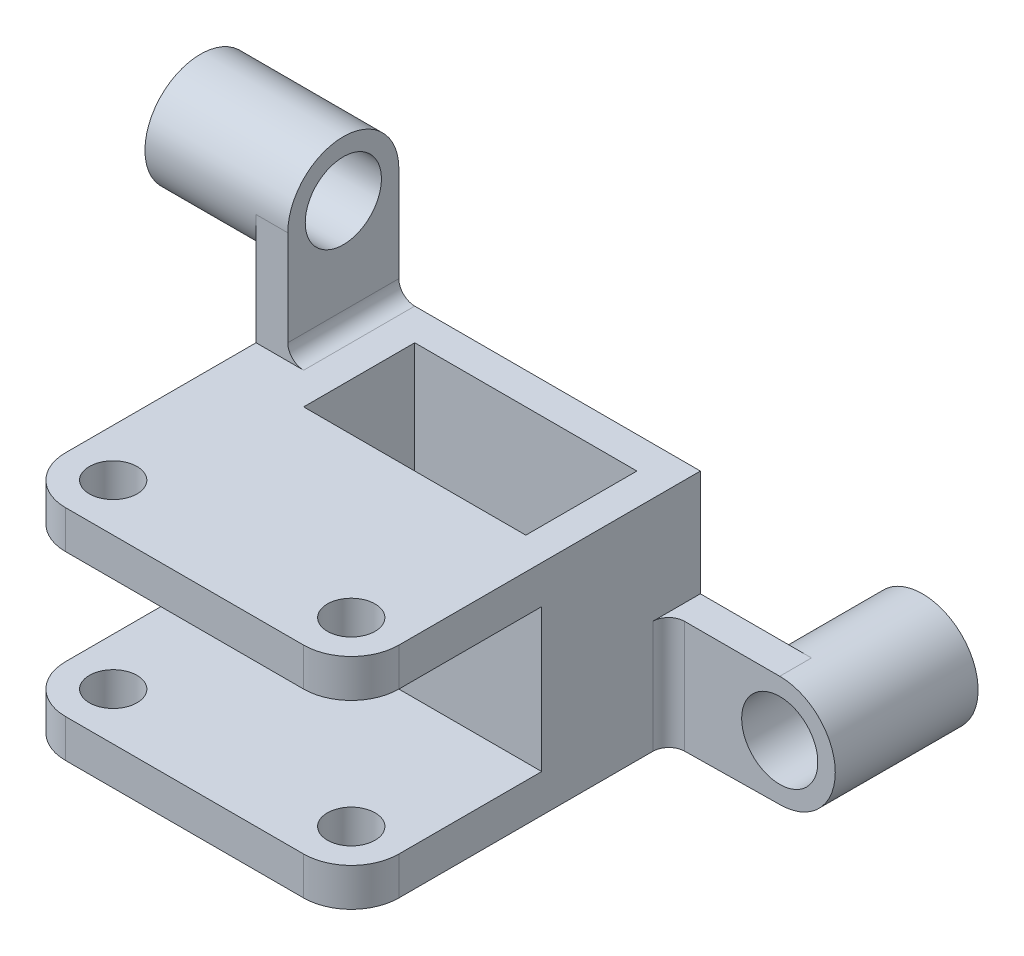
ISO-10303-21;
HEADER;
FILE_DESCRIPTION(('STEP AP214'),'2;1');
FILE_NAME('part.step','',(''),(''),'','','');
FILE_SCHEMA(('AUTOMOTIVE_DESIGN { 1 0 10303 214 1 1 1 1 }'));
ENDSEC;
DATA;
#1=APPLICATION_CONTEXT('core data for automotive mechanical design processes');
#2=APPLICATION_PROTOCOL_DEFINITION('international standard','automotive_design',2000,#1);
#3=PRODUCT_CONTEXT('',#1,'mechanical');
#4=PRODUCT('Part','Part','',(#3));
#5=PRODUCT_RELATED_PRODUCT_CATEGORY('part','',(#4));
#6=PRODUCT_DEFINITION_FORMATION('','',#4);
#7=PRODUCT_DEFINITION_CONTEXT('part definition',#1,'design');
#8=PRODUCT_DEFINITION('design','',#6,#7);
#9=PRODUCT_DEFINITION_SHAPE('','',#8);
#10=(LENGTH_UNIT() NAMED_UNIT(*) SI_UNIT(.MILLI.,.METRE.));
#11=(NAMED_UNIT(*) PLANE_ANGLE_UNIT() SI_UNIT($,.RADIAN.));
#12=(NAMED_UNIT(*) SI_UNIT($,.STERADIAN.) SOLID_ANGLE_UNIT());
#13=UNCERTAINTY_MEASURE_WITH_UNIT(LENGTH_MEASURE(1.E-05),#10,'distance_accuracy_value','');
#14=(GEOMETRIC_REPRESENTATION_CONTEXT(3) GLOBAL_UNCERTAINTY_ASSIGNED_CONTEXT((#13)) GLOBAL_UNIT_ASSIGNED_CONTEXT((#10,
#11,#12)) REPRESENTATION_CONTEXT('',''));
#15=CARTESIAN_POINT('',(0.,0.,0.));
#16=DIRECTION('',(0.,0.,1.));
#17=DIRECTION('',(1.,0.,0.));
#18=AXIS2_PLACEMENT_3D('',#15,#16,#17);
#19=CARTESIAN_POINT('',(-52.5,69.,55.));
#20=DIRECTION('',(1.,0.,0.));
#21=DIRECTION('',(0.,0.,-1.));
#22=AXIS2_PLACEMENT_3D('',#19,#20,#21);
#23=PLANE('',#22);
#24=CARTESIAN_POINT('',(-52.5,104.,-37.5));
#25=DIRECTION('',(-1.,0.,0.));
#26=DIRECTION('',(0.,0.,1.));
#27=AXIS2_PLACEMENT_3D('',#24,#25,#26);
#28=CIRCLE('',#27,17.5);
#29=CARTESIAN_POINT('',(-52.5,104.,-55.));
#30=VERTEX_POINT('',#29);
#31=CARTESIAN_POINT('',(-52.5,104.,-20.));
#32=VERTEX_POINT('',#31);
#33=EDGE_CURVE('E220',#30,#32,#28,.T.);
#34=ORIENTED_EDGE('',*,*,#33,.F.);
#35=DIRECTION('',(0.,-1.,0.));
#36=VECTOR('',#35,1.);
#37=CARTESIAN_POINT('',(-52.5,69.,-55.));
#38=LINE('',#37,#36);
#39=CARTESIAN_POINT('',(-52.5,0.,-55.));
#40=VERTEX_POINT('',#39);
#41=EDGE_CURVE('E224',#30,#40,#38,.T.);
#42=ORIENTED_EDGE('',*,*,#41,.T.);
#43=DIRECTION('',(0.,0.,1.));
#44=VECTOR('',#43,1.);
#45=CARTESIAN_POINT('',(-52.5,0.,55.));
#46=LINE('',#45,#44);
#47=CARTESIAN_POINT('',(-52.5,0.,40.));
#48=VERTEX_POINT('',#47);
#49=EDGE_CURVE('E383',#40,#48,#46,.T.);
#50=ORIENTED_EDGE('',*,*,#49,.T.);
#51=DIRECTION('',(0.,-1.,0.));
#52=VECTOR('',#51,1.);
#53=CARTESIAN_POINT('',(-52.5,69.,40.));
#54=LINE('',#53,#52);
#55=CARTESIAN_POINT('',(-52.5,12.,40.));
#56=VERTEX_POINT('',#55);
#57=EDGE_CURVE('E399',#48,#56,#54,.F.);
#58=ORIENTED_EDGE('',*,*,#57,.T.);
#59=DIRECTION('',(0.,0.,1.));
#60=VECTOR('',#59,1.);
#61=CARTESIAN_POINT('',(-52.5,12.,-4.99999999999999));
#62=LINE('',#61,#60);
#63=CARTESIAN_POINT('',(-52.5,12.,-4.99999999999999));
#64=VERTEX_POINT('',#63);
#65=EDGE_CURVE('E358',#64,#56,#62,.T.);
#66=ORIENTED_EDGE('',*,*,#65,.F.);
#67=DIRECTION('',(0.,-1.,0.));
#68=VECTOR('',#67,1.);
#69=CARTESIAN_POINT('',(-52.5,57.,-4.99999999999999));
#70=LINE('',#69,#68);
#71=CARTESIAN_POINT('',(-52.5,57.,-4.99999999999999));
#72=VERTEX_POINT('',#71);
#73=EDGE_CURVE('E343',#72,#64,#70,.T.);
#74=ORIENTED_EDGE('',*,*,#73,.F.);
#75=DIRECTION('',(0.,0.,1.));
#76=VECTOR('',#75,1.);
#77=CARTESIAN_POINT('',(-52.5,57.,-4.99999999999999));
#78=LINE('',#77,#76);
#79=CARTESIAN_POINT('',(-52.5,57.,40.));
#80=VERTEX_POINT('',#79);
#81=EDGE_CURVE('E363',#72,#80,#78,.T.);
#82=ORIENTED_EDGE('',*,*,#81,.T.);
#83=DIRECTION('',(0.,-1.,0.));
#84=VECTOR('',#83,1.);
#85=CARTESIAN_POINT('',(-52.5,69.,40.));
#86=LINE('',#85,#84);
#87=CARTESIAN_POINT('',(-52.5,69.,40.));
#88=VERTEX_POINT('',#87);
#89=EDGE_CURVE('E405',#80,#88,#86,.F.);
#90=ORIENTED_EDGE('',*,*,#89,.T.);
#91=DIRECTION('',(0.,0.,1.));
#92=VECTOR('',#91,1.);
#93=CARTESIAN_POINT('',(-52.5,69.,55.));
#94=LINE('',#93,#92);
#95=CARTESIAN_POINT('',(-52.5,69.,-20.));
#96=VERTEX_POINT('',#95);
#97=EDGE_CURVE('E378',#96,#88,#94,.T.);
#98=ORIENTED_EDGE('',*,*,#97,.F.);
#99=DIRECTION('',(0.,1.,0.));
#100=VECTOR('',#99,1.);
#101=CARTESIAN_POINT('',(-52.5,69.,-20.));
#102=LINE('',#101,#100);
#103=EDGE_CURVE('E240',#96,#32,#102,.T.);
#104=ORIENTED_EDGE('',*,*,#103,.T.);
#105=EDGE_LOOP('',(#34,#42,#50,#58,#66,#74,#82,#90,#98,#104));
#106=FACE_BOUND('',#105,.T.);
#107=ADVANCED_FACE('F44',(#106),#23,.F.);
#108=CARTESIAN_POINT('',(-52.5,69.,55.));
#109=DIRECTION('',(0.,0.,-1.));
#110=DIRECTION('',(-1.,0.,0.));
#111=AXIS2_PLACEMENT_3D('',#108,#109,#110);
#112=PLANE('',#111);
#113=DIRECTION('',(1.,0.,0.));
#114=VECTOR('',#113,1.);
#115=CARTESIAN_POINT('',(-52.5,69.,55.));
#116=LINE('',#115,#114);
#117=CARTESIAN_POINT('',(-37.5,69.,55.));
#118=VERTEX_POINT('',#117);
#119=CARTESIAN_POINT('',(37.5,69.,55.));
#120=VERTEX_POINT('',#119);
#121=EDGE_CURVE('E231',#118,#120,#116,.T.);
#122=ORIENTED_EDGE('',*,*,#121,.F.);
#123=DIRECTION('',(0.,-1.,0.));
#124=VECTOR('',#123,1.);
#125=CARTESIAN_POINT('',(-37.5,69.,55.));
#126=LINE('',#125,#124);
#127=CARTESIAN_POINT('',(-37.5,57.,55.));
#128=VERTEX_POINT('',#127);
#129=EDGE_CURVE('E392',#118,#128,#126,.T.);
#130=ORIENTED_EDGE('',*,*,#129,.T.);
#131=DIRECTION('',(-1.,0.,0.));
#132=VECTOR('',#131,1.);
#133=CARTESIAN_POINT('',(-52.5,57.,55.));
#134=LINE('',#133,#132);
#135=CARTESIAN_POINT('',(37.5,57.,55.));
#136=VERTEX_POINT('',#135);
#137=EDGE_CURVE('E347',#136,#128,#134,.T.);
#138=ORIENTED_EDGE('',*,*,#137,.F.);
#139=DIRECTION('',(0.,-1.,0.));
#140=VECTOR('',#139,1.);
#141=CARTESIAN_POINT('',(37.5,69.,55.));
#142=LINE('',#141,#140);
#143=EDGE_CURVE('E391',#136,#120,#142,.F.);
#144=ORIENTED_EDGE('',*,*,#143,.T.);
#145=EDGE_LOOP('',(#122,#130,#138,#144));
#146=FACE_BOUND('',#145,.T.);
#147=ADVANCED_FACE('F469',(#146),#112,.F.);
#148=CARTESIAN_POINT('',(52.5,69.,55.));
#149=DIRECTION('',(-1.,0.,0.));
#150=DIRECTION('',(0.,0.,1.));
#151=AXIS2_PLACEMENT_3D('',#148,#149,#150);
#152=PLANE('',#151);
#153=DIRECTION('',(0.,0.,-1.));
#154=VECTOR('',#153,1.);
#155=CARTESIAN_POINT('',(52.5,0.,55.));
#156=LINE('',#155,#154);
#157=CARTESIAN_POINT('',(52.5,0.,40.));
#158=VERTEX_POINT('',#157);
#159=CARTESIAN_POINT('',(52.5,0.,-40.));
#160=VERTEX_POINT('',#159);
#161=EDGE_CURVE('E364',#158,#160,#156,.T.);
#162=ORIENTED_EDGE('',*,*,#161,.T.);
#163=DIRECTION('',(0.,1.,0.));
#164=VECTOR('',#163,1.);
#165=CARTESIAN_POINT('',(52.5,35.5,-40.));
#166=LINE('',#165,#164);
#167=CARTESIAN_POINT('',(52.5,35.5,-40.));
#168=VERTEX_POINT('',#167);
#169=EDGE_CURVE('E267',#160,#168,#166,.T.);
#170=ORIENTED_EDGE('',*,*,#169,.T.);
#171=DIRECTION('',(0.,0.,-1.));
#172=VECTOR('',#171,1.);
#173=CARTESIAN_POINT('',(52.5,35.5,-45.));
#174=LINE('',#173,#172);
#175=CARTESIAN_POINT('',(52.5,35.5,-55.));
#176=VERTEX_POINT('',#175);
#177=EDGE_CURVE('E290',#168,#176,#174,.T.);
#178=ORIENTED_EDGE('',*,*,#177,.T.);
#179=DIRECTION('',(0.,-1.,0.));
#180=VECTOR('',#179,1.);
#181=CARTESIAN_POINT('',(52.5,69.,-55.));
#182=LINE('',#181,#180);
#183=CARTESIAN_POINT('',(52.5,69.,-55.));
#184=VERTEX_POINT('',#183);
#185=EDGE_CURVE('E235',#184,#176,#182,.T.);
#186=ORIENTED_EDGE('',*,*,#185,.F.);
#187=DIRECTION('',(0.,0.,-1.));
#188=VECTOR('',#187,1.);
#189=CARTESIAN_POINT('',(52.5,69.,55.));
#190=LINE('',#189,#188);
#191=CARTESIAN_POINT('',(52.5,69.,40.));
#192=VERTEX_POINT('',#191);
#193=EDGE_CURVE('E373',#192,#184,#190,.T.);
#194=ORIENTED_EDGE('',*,*,#193,.F.);
#195=DIRECTION('',(0.,-1.,0.));
#196=VECTOR('',#195,1.);
#197=CARTESIAN_POINT('',(52.5,69.,40.));
#198=LINE('',#197,#196);
#199=CARTESIAN_POINT('',(52.5,57.,40.));
#200=VERTEX_POINT('',#199);
#201=EDGE_CURVE('E422',#192,#200,#198,.T.);
#202=ORIENTED_EDGE('',*,*,#201,.T.);
#203=DIRECTION('',(0.,0.,1.));
#204=VECTOR('',#203,1.);
#205=CARTESIAN_POINT('',(52.5,57.,-4.99999999999999));
#206=LINE('',#205,#204);
#207=CARTESIAN_POINT('',(52.5,57.,-4.99999999999999));
#208=VERTEX_POINT('',#207);
#209=EDGE_CURVE('E362',#208,#200,#206,.T.);
#210=ORIENTED_EDGE('',*,*,#209,.F.);
#211=DIRECTION('',(0.,1.,0.));
#212=VECTOR('',#211,1.);
#213=CARTESIAN_POINT('',(52.5,57.,-4.99999999999999));
#214=LINE('',#213,#212);
#215=CARTESIAN_POINT('',(52.5,12.,-4.99999999999999));
#216=VERTEX_POINT('',#215);
#217=EDGE_CURVE('E351',#216,#208,#214,.T.);
#218=ORIENTED_EDGE('',*,*,#217,.F.);
#219=DIRECTION('',(0.,0.,1.));
#220=VECTOR('',#219,1.);
#221=CARTESIAN_POINT('',(52.5,12.,-4.99999999999999));
#222=LINE('',#221,#220);
#223=CARTESIAN_POINT('',(52.5,12.,40.));
#224=VERTEX_POINT('',#223);
#225=EDGE_CURVE('E368',#216,#224,#222,.T.);
#226=ORIENTED_EDGE('',*,*,#225,.T.);
#227=DIRECTION('',(0.,-1.,0.));
#228=VECTOR('',#227,1.);
#229=CARTESIAN_POINT('',(52.5,69.,40.));
#230=LINE('',#229,#228);
#231=EDGE_CURVE('E269',#224,#158,#230,.T.);
#232=ORIENTED_EDGE('',*,*,#231,.T.);
#233=EDGE_LOOP('',(#162,#170,#178,#186,#194,#202,#210,#218,#226,#232));
#234=FACE_BOUND('',#233,.T.);
#235=ADVANCED_FACE('F457',(#234),#152,.F.);
#236=CARTESIAN_POINT('',(-52.5,69.,-55.));
#237=DIRECTION('',(0.,0.,1.));
#238=DIRECTION('',(1.,0.,0.));
#239=AXIS2_PLACEMENT_3D('',#236,#237,#238);
#240=PLANE('',#239);
#241=CARTESIAN_POINT('',(87.5,18.,-55.));
#242=DIRECTION('',(0.,0.,-1.));
#243=DIRECTION('',(-1.,0.,0.));
#244=AXIS2_PLACEMENT_3D('',#241,#242,#243);
#245=CIRCLE('',#244,17.5);
#246=CARTESIAN_POINT('',(87.5,0.499999999999997,-55.));
#247=VERTEX_POINT('',#246);
#248=CARTESIAN_POINT('',(87.5,35.5,-55.));
#249=VERTEX_POINT('',#248);
#250=EDGE_CURVE('E266',#247,#249,#245,.T.);
#251=ORIENTED_EDGE('',*,*,#250,.F.);
#252=DIRECTION('',(-0.99989797479951,-0.0142842567828501,0.));
#253=VECTOR('',#252,1.);
#254=CARTESIAN_POINT('',(87.5,0.499999999999997,-55.));
#255=LINE('',#254,#253);
#256=CARTESIAN_POINT('',(52.5,0.,-55.));
#257=VERTEX_POINT('',#256);
#258=EDGE_CURVE('E264',#247,#257,#255,.T.);
#259=ORIENTED_EDGE('',*,*,#258,.T.);
#260=DIRECTION('',(-1.,0.,0.));
#261=VECTOR('',#260,1.);
#262=CARTESIAN_POINT('',(-52.5,0.,-55.));
#263=LINE('',#262,#261);
#264=EDGE_CURVE('E226',#257,#40,#263,.T.);
#265=ORIENTED_EDGE('',*,*,#264,.T.);
#266=ORIENTED_EDGE('',*,*,#41,.F.);
#267=DIRECTION('',(-1.,0.,0.));
#268=VECTOR('',#267,1.);
#269=CARTESIAN_POINT('',(-42.5,104.,-55.));
#270=LINE('',#269,#268);
#271=CARTESIAN_POINT('',(-42.5,104.,-55.));
#272=VERTEX_POINT('',#271);
#273=EDGE_CURVE('E214',#272,#30,#270,.T.);
#274=ORIENTED_EDGE('',*,*,#273,.F.);
#275=DIRECTION('',(0.,-1.,0.));
#276=VECTOR('',#275,1.);
#277=CARTESIAN_POINT('',(-42.5,104.,-55.));
#278=LINE('',#277,#276);
#279=CARTESIAN_POINT('',(-42.5,74.,-55.));
#280=VERTEX_POINT('',#279);
#281=EDGE_CURVE('E247',#272,#280,#278,.T.);
#282=ORIENTED_EDGE('',*,*,#281,.T.);
#283=CARTESIAN_POINT('',(-37.5,74.,-55.));
#284=DIRECTION('',(0.,0.,1.));
#285=DIRECTION('',(1.,0.,0.));
#286=AXIS2_PLACEMENT_3D('',#283,#284,#285);
#287=CIRCLE('',#286,5.);
#288=CARTESIAN_POINT('',(-37.5,69.,-55.));
#289=VERTEX_POINT('',#288);
#290=EDGE_CURVE('E11',#280,#289,#287,.T.);
#291=ORIENTED_EDGE('',*,*,#290,.T.);
#292=DIRECTION('',(-1.,0.,0.));
#293=VECTOR('',#292,1.);
#294=CARTESIAN_POINT('',(-52.5,69.,-55.));
#295=LINE('',#294,#293);
#296=EDGE_CURVE('E374',#184,#289,#295,.T.);
#297=ORIENTED_EDGE('',*,*,#296,.F.);
#298=ORIENTED_EDGE('',*,*,#185,.T.);
#299=DIRECTION('',(1.,0.,0.));
#300=VECTOR('',#299,1.);
#301=CARTESIAN_POINT('',(52.5,35.5,-55.));
#302=LINE('',#301,#300);
#303=EDGE_CURVE('E273',#176,#249,#302,.T.);
#304=ORIENTED_EDGE('',*,*,#303,.T.);
#305=EDGE_LOOP('',(#251,#259,#265,#266,#274,#282,#291,#297,#298,#304));
#306=FACE_BOUND('',#305,.T.);
#307=ADVANCED_FACE('F228',(#306),#240,.F.);
#308=DIRECTION('',(1.,0.,0.));
#309=VECTOR('',#308,1.);
#310=CARTESIAN_POINT('',(-52.5,12.,55.));
#311=LINE('',#310,#309);
#312=CARTESIAN_POINT('',(-37.5,12.,55.));
#313=VERTEX_POINT('',#312);
#314=CARTESIAN_POINT('',(37.5,12.,55.));
#315=VERTEX_POINT('',#314);
#316=EDGE_CURVE('E345',#313,#315,#311,.T.);
#317=ORIENTED_EDGE('',*,*,#316,.F.);
#318=DIRECTION('',(0.,-1.,0.));
#319=VECTOR('',#318,1.);
#320=CARTESIAN_POINT('',(-37.5,69.,55.));
#321=LINE('',#320,#319);
#322=CARTESIAN_POINT('',(-37.5,0.,55.));
#323=VERTEX_POINT('',#322);
#324=EDGE_CURVE('E411',#313,#323,#321,.T.);
#325=ORIENTED_EDGE('',*,*,#324,.T.);
#326=DIRECTION('',(1.,0.,0.));
#327=VECTOR('',#326,1.);
#328=CARTESIAN_POINT('',(-52.5,0.,55.));
#329=LINE('',#328,#327);
#330=CARTESIAN_POINT('',(37.5,0.,55.));
#331=VERTEX_POINT('',#330);
#332=EDGE_CURVE('E376',#323,#331,#329,.T.);
#333=ORIENTED_EDGE('',*,*,#332,.T.);
#334=DIRECTION('',(0.,-1.,0.));
#335=VECTOR('',#334,1.);
#336=CARTESIAN_POINT('',(37.5,69.,55.));
#337=LINE('',#336,#335);
#338=EDGE_CURVE('E408',#331,#315,#337,.F.);
#339=ORIENTED_EDGE('',*,*,#338,.T.);
#340=EDGE_LOOP('',(#317,#325,#333,#339));
#341=FACE_BOUND('',#340,.T.);
#342=ADVANCED_FACE('F489',(#341),#112,.F.);
#343=CARTESIAN_POINT('',(0.,69.,0.));
#344=DIRECTION('',(0.,-1.,0.));
#345=DIRECTION('',(0.,0.,-1.));
#346=AXIS2_PLACEMENT_3D('',#343,#344,#345);
#347=PLANE('',#346);
#348=DIRECTION('',(1.,0.,0.));
#349=VECTOR('',#348,1.);
#350=CARTESIAN_POINT('',(-27.5,69.,-9.99999999999999));
#351=LINE('',#350,#349);
#352=CARTESIAN_POINT('',(-27.5,69.,-9.99999999999999));
#353=VERTEX_POINT('',#352);
#354=CARTESIAN_POINT('',(42.5,69.,-9.99999999999999));
#355=VERTEX_POINT('',#354);
#356=EDGE_CURVE('E310',#353,#355,#351,.T.);
#357=ORIENTED_EDGE('',*,*,#356,.F.);
#358=DIRECTION('',(0.,0.,1.));
#359=VECTOR('',#358,1.);
#360=CARTESIAN_POINT('',(-27.5,69.,-45.));
#361=LINE('',#360,#359);
#362=CARTESIAN_POINT('',(-27.5,69.,-45.));
#363=VERTEX_POINT('',#362);
#364=EDGE_CURVE('E286',#363,#353,#361,.T.);
#365=ORIENTED_EDGE('',*,*,#364,.F.);
#366=DIRECTION('',(-1.,0.,0.));
#367=VECTOR('',#366,1.);
#368=CARTESIAN_POINT('',(-27.5,69.,-45.));
#369=LINE('',#368,#367);
#370=CARTESIAN_POINT('',(42.5,69.,-45.));
#371=VERTEX_POINT('',#370);
#372=EDGE_CURVE('E298',#371,#363,#369,.T.);
#373=ORIENTED_EDGE('',*,*,#372,.F.);
#374=DIRECTION('',(0.,0.,-1.));
#375=VECTOR('',#374,1.);
#376=CARTESIAN_POINT('',(42.5,69.,-45.));
#377=LINE('',#376,#375);
#378=EDGE_CURVE('E309',#355,#371,#377,.T.);
#379=ORIENTED_EDGE('',*,*,#378,.F.);
#380=EDGE_LOOP('',(#357,#365,#373,#379));
#381=FACE_BOUND('',#380,.T.);
#382=CARTESIAN_POINT('',(-37.5,69.,40.));
#383=DIRECTION('',(0.,1.,0.));
#384=DIRECTION('',(0.,0.,1.));
#385=AXIS2_PLACEMENT_3D('',#382,#383,#384);
#386=CIRCLE('',#385,7.5);
#387=CARTESIAN_POINT('',(-37.5,69.,47.5));
#388=VERTEX_POINT('',#387);
#389=EDGE_CURVE('E327',#388,#388,#386,.T.);
#390=ORIENTED_EDGE('',*,*,#389,.F.);
#391=EDGE_LOOP('',(#390));
#392=FACE_BOUND('',#391,.T.);
#393=CARTESIAN_POINT('',(37.5,69.,40.));
#394=DIRECTION('',(0.,1.,0.));
#395=DIRECTION('',(0.,0.,1.));
#396=AXIS2_PLACEMENT_3D('',#393,#394,#395);
#397=CIRCLE('',#396,7.5);
#398=CARTESIAN_POINT('',(37.5,69.,47.5));
#399=VERTEX_POINT('',#398);
#400=EDGE_CURVE('E320',#399,#399,#397,.T.);
#401=ORIENTED_EDGE('',*,*,#400,.F.);
#402=EDGE_LOOP('',(#401));
#403=FACE_BOUND('',#402,.T.);
#404=ORIENTED_EDGE('',*,*,#296,.T.);
#405=DIRECTION('',(0.,0.,1.));
#406=VECTOR('',#405,1.);
#407=CARTESIAN_POINT('',(-37.5,69.,-20.));
#408=LINE('',#407,#406);
#409=CARTESIAN_POINT('',(-37.5,69.,-20.));
#410=VERTEX_POINT('',#409);
#411=EDGE_CURVE('E434',#289,#410,#408,.T.);
#412=ORIENTED_EDGE('',*,*,#411,.T.);
#413=DIRECTION('',(-1.,0.,0.));
#414=VECTOR('',#413,1.);
#415=CARTESIAN_POINT('',(-42.5,69.,-20.));
#416=LINE('',#415,#414);
#417=EDGE_CURVE('E221',#410,#96,#416,.T.);
#418=ORIENTED_EDGE('',*,*,#417,.T.);
#419=ORIENTED_EDGE('',*,*,#97,.T.);
#420=CARTESIAN_POINT('',(-37.5,69.,40.));
#421=DIRECTION('',(0.,-1.,0.));
#422=DIRECTION('',(0.,0.,-1.));
#423=AXIS2_PLACEMENT_3D('',#420,#421,#422);
#424=CIRCLE('',#423,15.);
#425=EDGE_CURVE('E406',#88,#118,#424,.F.);
#426=ORIENTED_EDGE('',*,*,#425,.T.);
#427=ORIENTED_EDGE('',*,*,#121,.T.);
#428=CARTESIAN_POINT('',(37.5,69.,40.));
#429=DIRECTION('',(0.,-1.,0.));
#430=DIRECTION('',(0.,0.,-1.));
#431=AXIS2_PLACEMENT_3D('',#428,#429,#430);
#432=CIRCLE('',#431,15.);
#433=EDGE_CURVE('E403',#120,#192,#432,.F.);
#434=ORIENTED_EDGE('',*,*,#433,.T.);
#435=ORIENTED_EDGE('',*,*,#193,.T.);
#436=EDGE_LOOP('',(#404,#412,#418,#419,#426,#427,#434,#435));
#437=FACE_BOUND('',#436,.T.);
#438=ADVANCED_FACE('F455',(#381,#392,#403,#437),#347,.F.);
#439=CARTESIAN_POINT('',(0.,0.,0.));
#440=DIRECTION('',(0.,-1.,0.));
#441=DIRECTION('',(0.,0.,-1.));
#442=AXIS2_PLACEMENT_3D('',#439,#440,#441);
#443=PLANE('',#442);
#444=DIRECTION('',(0.,0.,1.));
#445=VECTOR('',#444,1.);
#446=CARTESIAN_POINT('',(-27.5,0.,-45.));
#447=LINE('',#446,#445);
#448=CARTESIAN_POINT('',(-27.5,0.,-45.));
#449=VERTEX_POINT('',#448);
#450=CARTESIAN_POINT('',(-27.5,0.,-9.99999999999999));
#451=VERTEX_POINT('',#450);
#452=EDGE_CURVE('E292',#449,#451,#447,.T.);
#453=ORIENTED_EDGE('',*,*,#452,.T.);
#454=DIRECTION('',(1.,0.,0.));
#455=VECTOR('',#454,1.);
#456=CARTESIAN_POINT('',(-27.5,0.,-9.99999999999999));
#457=LINE('',#456,#455);
#458=CARTESIAN_POINT('',(42.5,0.,-9.99999999999999));
#459=VERTEX_POINT('',#458);
#460=EDGE_CURVE('E294',#451,#459,#457,.T.);
#461=ORIENTED_EDGE('',*,*,#460,.T.);
#462=DIRECTION('',(0.,0.,-1.));
#463=VECTOR('',#462,1.);
#464=CARTESIAN_POINT('',(42.5,0.,-45.));
#465=LINE('',#464,#463);
#466=CARTESIAN_POINT('',(42.5,0.,-45.));
#467=VERTEX_POINT('',#466);
#468=EDGE_CURVE('E299',#459,#467,#465,.T.);
#469=ORIENTED_EDGE('',*,*,#468,.T.);
#470=DIRECTION('',(-1.,0.,0.));
#471=VECTOR('',#470,1.);
#472=CARTESIAN_POINT('',(-27.5,0.,-45.));
#473=LINE('',#472,#471);
#474=EDGE_CURVE('E305',#467,#449,#473,.T.);
#475=ORIENTED_EDGE('',*,*,#474,.T.);
#476=EDGE_LOOP('',(#453,#461,#469,#475));
#477=FACE_BOUND('',#476,.T.);
#478=CARTESIAN_POINT('',(-37.5,0.,40.));
#479=DIRECTION('',(0.,1.,0.));
#480=DIRECTION('',(0.,0.,1.));
#481=AXIS2_PLACEMENT_3D('',#478,#479,#480);
#482=CIRCLE('',#481,7.5);
#483=CARTESIAN_POINT('',(-37.5,0.,47.5));
#484=VERTEX_POINT('',#483);
#485=EDGE_CURVE('E323',#484,#484,#482,.T.);
#486=ORIENTED_EDGE('',*,*,#485,.T.);
#487=EDGE_LOOP('',(#486));
#488=FACE_BOUND('',#487,.T.);
#489=CARTESIAN_POINT('',(37.5,0.,40.));
#490=DIRECTION('',(0.,1.,0.));
#491=DIRECTION('',(0.,0.,1.));
#492=AXIS2_PLACEMENT_3D('',#489,#490,#491);
#493=CIRCLE('',#492,7.5);
#494=CARTESIAN_POINT('',(37.5,0.,47.5));
#495=VERTEX_POINT('',#494);
#496=EDGE_CURVE('E331',#495,#495,#493,.T.);
#497=ORIENTED_EDGE('',*,*,#496,.T.);
#498=EDGE_LOOP('',(#497));
#499=FACE_BOUND('',#498,.T.);
#500=ORIENTED_EDGE('',*,*,#332,.F.);
#501=CARTESIAN_POINT('',(-37.5,0.,40.));
#502=DIRECTION('',(0.,-1.,0.));
#503=DIRECTION('',(0.,0.,-1.));
#504=AXIS2_PLACEMENT_3D('',#501,#502,#503);
#505=CIRCLE('',#504,15.);
#506=EDGE_CURVE('E416',#323,#48,#505,.T.);
#507=ORIENTED_EDGE('',*,*,#506,.T.);
#508=ORIENTED_EDGE('',*,*,#49,.F.);
#509=ORIENTED_EDGE('',*,*,#264,.F.);
#510=DIRECTION('',(0.,0.,-1.));
#511=VECTOR('',#510,1.);
#512=CARTESIAN_POINT('',(52.5,0.,-45.));
#513=LINE('',#512,#511);
#514=EDGE_CURVE('E58',#160,#257,#513,.T.);
#515=ORIENTED_EDGE('',*,*,#514,.F.);
#516=ORIENTED_EDGE('',*,*,#161,.F.);
#517=CARTESIAN_POINT('',(37.5,0.,40.));
#518=DIRECTION('',(0.,-1.,0.));
#519=DIRECTION('',(0.,0.,-1.));
#520=AXIS2_PLACEMENT_3D('',#517,#518,#519);
#521=CIRCLE('',#520,15.);
#522=EDGE_CURVE('E413',#158,#331,#521,.T.);
#523=ORIENTED_EDGE('',*,*,#522,.T.);
#524=EDGE_LOOP('',(#500,#507,#508,#509,#515,#516,#523));
#525=FACE_BOUND('',#524,.T.);
#526=ADVANCED_FACE('F487',(#477,#488,#499,#525),#443,.T.);
#527=CARTESIAN_POINT('',(-52.5,57.,-4.99999999999999));
#528=DIRECTION('',(0.,1.,0.));
#529=DIRECTION('',(0.,0.,1.));
#530=AXIS2_PLACEMENT_3D('',#527,#528,#529);
#531=PLANE('',#530);
#532=CARTESIAN_POINT('',(-37.5,57.,40.));
#533=DIRECTION('',(0.,1.,0.));
#534=DIRECTION('',(0.,0.,1.));
#535=AXIS2_PLACEMENT_3D('',#532,#533,#534);
#536=CIRCLE('',#535,7.5);
#537=CARTESIAN_POINT('',(-37.5,57.,47.5));
#538=VERTEX_POINT('',#537);
#539=EDGE_CURVE('E338',#538,#538,#536,.T.);
#540=ORIENTED_EDGE('',*,*,#539,.T.);
#541=EDGE_LOOP('',(#540));
#542=FACE_BOUND('',#541,.T.);
#543=CARTESIAN_POINT('',(37.5,57.,40.));
#544=DIRECTION('',(0.,1.,0.));
#545=DIRECTION('',(0.,0.,1.));
#546=AXIS2_PLACEMENT_3D('',#543,#544,#545);
#547=CIRCLE('',#546,7.5);
#548=CARTESIAN_POINT('',(37.5,57.,47.5));
#549=VERTEX_POINT('',#548);
#550=EDGE_CURVE('E337',#549,#549,#547,.T.);
#551=ORIENTED_EDGE('',*,*,#550,.T.);
#552=EDGE_LOOP('',(#551));
#553=FACE_BOUND('',#552,.T.);
#554=ORIENTED_EDGE('',*,*,#137,.T.);
#555=CARTESIAN_POINT('',(-37.5,57.,40.));
#556=DIRECTION('',(0.,1.,0.));
#557=DIRECTION('',(0.,0.,1.));
#558=AXIS2_PLACEMENT_3D('',#555,#556,#557);
#559=CIRCLE('',#558,15.);
#560=EDGE_CURVE('E398',#128,#80,#559,.F.);
#561=ORIENTED_EDGE('',*,*,#560,.T.);
#562=ORIENTED_EDGE('',*,*,#81,.F.);
#563=DIRECTION('',(-1.,0.,0.));
#564=VECTOR('',#563,1.);
#565=CARTESIAN_POINT('',(-52.5,57.,-4.99999999999999));
#566=LINE('',#565,#564);
#567=EDGE_CURVE('E353',#208,#72,#566,.T.);
#568=ORIENTED_EDGE('',*,*,#567,.F.);
#569=ORIENTED_EDGE('',*,*,#209,.T.);
#570=CARTESIAN_POINT('',(37.5,57.,40.));
#571=DIRECTION('',(0.,1.,0.));
#572=DIRECTION('',(0.,0.,1.));
#573=AXIS2_PLACEMENT_3D('',#570,#571,#572);
#574=CIRCLE('',#573,15.);
#575=EDGE_CURVE('E396',#200,#136,#574,.F.);
#576=ORIENTED_EDGE('',*,*,#575,.T.);
#577=EDGE_LOOP('',(#554,#561,#562,#568,#569,#576));
#578=FACE_BOUND('',#577,.T.);
#579=ADVANCED_FACE('F464',(#542,#553,#578),#531,.F.);
#580=CARTESIAN_POINT('',(-52.5,12.,-4.99999999999999));
#581=DIRECTION('',(0.,-1.,0.));
#582=DIRECTION('',(1.,0.,0.));
#583=AXIS2_PLACEMENT_3D('',#580,#581,#582);
#584=PLANE('',#583);
#585=CARTESIAN_POINT('',(-37.5,12.,40.));
#586=DIRECTION('',(0.,-1.,0.));
#587=DIRECTION('',(1.,0.,0.));
#588=AXIS2_PLACEMENT_3D('',#585,#586,#587);
#589=CIRCLE('',#588,7.5);
#590=CARTESIAN_POINT('',(-30.,12.,40.));
#591=VERTEX_POINT('',#590);
#592=EDGE_CURVE('E339',#591,#591,#589,.T.);
#593=ORIENTED_EDGE('',*,*,#592,.T.);
#594=EDGE_LOOP('',(#593));
#595=FACE_BOUND('',#594,.T.);
#596=CARTESIAN_POINT('',(37.5,12.,40.));
#597=DIRECTION('',(0.,-1.,0.));
#598=DIRECTION('',(1.,0.,0.));
#599=AXIS2_PLACEMENT_3D('',#596,#597,#598);
#600=CIRCLE('',#599,7.5);
#601=CARTESIAN_POINT('',(45.,12.,40.));
#602=VERTEX_POINT('',#601);
#603=EDGE_CURVE('E330',#602,#602,#600,.T.);
#604=ORIENTED_EDGE('',*,*,#603,.T.);
#605=EDGE_LOOP('',(#604));
#606=FACE_BOUND('',#605,.T.);
#607=ORIENTED_EDGE('',*,*,#65,.T.);
#608=CARTESIAN_POINT('',(-37.5,12.,40.));
#609=DIRECTION('',(0.,-1.,0.));
#610=DIRECTION('',(1.,0.,0.));
#611=AXIS2_PLACEMENT_3D('',#608,#609,#610);
#612=CIRCLE('',#611,15.);
#613=EDGE_CURVE('E419',#56,#313,#612,.F.);
#614=ORIENTED_EDGE('',*,*,#613,.T.);
#615=ORIENTED_EDGE('',*,*,#316,.T.);
#616=CARTESIAN_POINT('',(37.5,12.,40.));
#617=DIRECTION('',(0.,-1.,0.));
#618=DIRECTION('',(1.,0.,0.));
#619=AXIS2_PLACEMENT_3D('',#616,#617,#618);
#620=CIRCLE('',#619,15.);
#621=EDGE_CURVE('E418',#315,#224,#620,.F.);
#622=ORIENTED_EDGE('',*,*,#621,.T.);
#623=ORIENTED_EDGE('',*,*,#225,.F.);
#624=DIRECTION('',(1.,0.,0.));
#625=VECTOR('',#624,1.);
#626=CARTESIAN_POINT('',(-52.5,12.,-4.99999999999999));
#627=LINE('',#626,#625);
#628=EDGE_CURVE('E350',#64,#216,#627,.T.);
#629=ORIENTED_EDGE('',*,*,#628,.F.);
#630=EDGE_LOOP('',(#607,#614,#615,#622,#623,#629));
#631=FACE_BOUND('',#630,.T.);
#632=ADVANCED_FACE('F496',(#595,#606,#631),#584,.F.);
#633=CARTESIAN_POINT('',(0.,0.,-4.99999999999999));
#634=DIRECTION('',(0.,0.,1.));
#635=DIRECTION('',(1.,0.,0.));
#636=AXIS2_PLACEMENT_3D('',#633,#634,#635);
#637=PLANE('',#636);
#638=ORIENTED_EDGE('',*,*,#73,.T.);
#639=ORIENTED_EDGE('',*,*,#628,.T.);
#640=ORIENTED_EDGE('',*,*,#217,.T.);
#641=ORIENTED_EDGE('',*,*,#567,.T.);
#642=EDGE_LOOP('',(#638,#639,#640,#641));
#643=FACE_BOUND('',#642,.T.);
#644=ADVANCED_FACE('F477',(#643),#637,.T.);
#645=CARTESIAN_POINT('',(-37.5,69.,40.));
#646=DIRECTION('',(0.,-1.,0.));
#647=DIRECTION('',(0.,0.,-1.));
#648=AXIS2_PLACEMENT_3D('',#645,#646,#647);
#649=CYLINDRICAL_SURFACE('',#648,15.);
#650=ORIENTED_EDGE('',*,*,#425,.F.);
#651=ORIENTED_EDGE('',*,*,#89,.F.);
#652=ORIENTED_EDGE('',*,*,#560,.F.);
#653=ORIENTED_EDGE('',*,*,#129,.F.);
#654=EDGE_LOOP('',(#650,#651,#652,#653));
#655=FACE_BOUND('',#654,.T.);
#656=ADVANCED_FACE('F475',(#655),#649,.T.);
#657=CARTESIAN_POINT('',(-37.5,69.,40.));
#658=DIRECTION('',(0.,-1.,0.));
#659=DIRECTION('',(0.,0.,-1.));
#660=AXIS2_PLACEMENT_3D('',#657,#658,#659);
#661=CYLINDRICAL_SURFACE('',#660,15.);
#662=ORIENTED_EDGE('',*,*,#613,.F.);
#663=ORIENTED_EDGE('',*,*,#57,.F.);
#664=ORIENTED_EDGE('',*,*,#506,.F.);
#665=ORIENTED_EDGE('',*,*,#324,.F.);
#666=EDGE_LOOP('',(#662,#663,#664,#665));
#667=FACE_BOUND('',#666,.T.);
#668=ADVANCED_FACE('F494',(#667),#661,.T.);
#669=CARTESIAN_POINT('',(37.5,69.,40.));
#670=DIRECTION('',(0.,-1.,0.));
#671=DIRECTION('',(0.,0.,-1.));
#672=AXIS2_PLACEMENT_3D('',#669,#670,#671);
#673=CYLINDRICAL_SURFACE('',#672,15.);
#674=ORIENTED_EDGE('',*,*,#621,.F.);
#675=ORIENTED_EDGE('',*,*,#338,.F.);
#676=ORIENTED_EDGE('',*,*,#522,.F.);
#677=ORIENTED_EDGE('',*,*,#231,.F.);
#678=EDGE_LOOP('',(#674,#675,#676,#677));
#679=FACE_BOUND('',#678,.T.);
#680=ADVANCED_FACE('F482',(#679),#673,.T.);
#681=CARTESIAN_POINT('',(37.5,69.,40.));
#682=DIRECTION('',(0.,-1.,0.));
#683=DIRECTION('',(0.,0.,-1.));
#684=AXIS2_PLACEMENT_3D('',#681,#682,#683);
#685=CYLINDRICAL_SURFACE('',#684,15.);
#686=ORIENTED_EDGE('',*,*,#433,.F.);
#687=ORIENTED_EDGE('',*,*,#143,.F.);
#688=ORIENTED_EDGE('',*,*,#575,.F.);
#689=ORIENTED_EDGE('',*,*,#201,.F.);
#690=EDGE_LOOP('',(#686,#687,#688,#689));
#691=FACE_BOUND('',#690,.T.);
#692=ADVANCED_FACE('F461',(#691),#685,.T.);
#693=CARTESIAN_POINT('',(37.5,0.,40.));
#694=DIRECTION('',(0.,1.,0.));
#695=DIRECTION('',(0.,0.,1.));
#696=AXIS2_PLACEMENT_3D('',#693,#694,#695);
#697=CYLINDRICAL_SURFACE('',#696,7.5);
#698=ORIENTED_EDGE('',*,*,#496,.F.);
#699=EDGE_LOOP('',(#698));
#700=FACE_BOUND('',#699,.T.);
#701=ORIENTED_EDGE('',*,*,#603,.F.);
#702=EDGE_LOOP('',(#701));
#703=FACE_BOUND('',#702,.T.);
#704=ADVANCED_FACE('F532',(#700,#703),#697,.F.);
#705=CARTESIAN_POINT('',(-37.5,0.,40.));
#706=DIRECTION('',(0.,1.,0.));
#707=DIRECTION('',(0.,0.,1.));
#708=AXIS2_PLACEMENT_3D('',#705,#706,#707);
#709=CYLINDRICAL_SURFACE('',#708,7.5);
#710=ORIENTED_EDGE('',*,*,#485,.F.);
#711=EDGE_LOOP('',(#710));
#712=FACE_BOUND('',#711,.T.);
#713=ORIENTED_EDGE('',*,*,#592,.F.);
#714=EDGE_LOOP('',(#713));
#715=FACE_BOUND('',#714,.T.);
#716=ADVANCED_FACE('F597',(#712,#715),#709,.F.);
#717=ORIENTED_EDGE('',*,*,#400,.T.);
#718=EDGE_LOOP('',(#717));
#719=FACE_BOUND('',#718,.T.);
#720=ORIENTED_EDGE('',*,*,#550,.F.);
#721=EDGE_LOOP('',(#720));
#722=FACE_BOUND('',#721,.T.);
#723=ADVANCED_FACE('F592',(#719,#722),#697,.F.);
#724=ORIENTED_EDGE('',*,*,#389,.T.);
#725=EDGE_LOOP('',(#724));
#726=FACE_BOUND('',#725,.T.);
#727=ORIENTED_EDGE('',*,*,#539,.F.);
#728=EDGE_LOOP('',(#727));
#729=FACE_BOUND('',#728,.T.);
#730=ADVANCED_FACE('F589',(#726,#729),#709,.F.);
#731=CARTESIAN_POINT('',(-27.5,0.,-45.));
#732=DIRECTION('',(-1.,0.,0.));
#733=DIRECTION('',(0.,0.,1.));
#734=AXIS2_PLACEMENT_3D('',#731,#732,#733);
#735=PLANE('',#734);
#736=ORIENTED_EDGE('',*,*,#364,.T.);
#737=DIRECTION('',(0.,1.,0.));
#738=VECTOR('',#737,1.);
#739=CARTESIAN_POINT('',(-27.5,0.,-9.99999999999999));
#740=LINE('',#739,#738);
#741=EDGE_CURVE('E304',#451,#353,#740,.T.);
#742=ORIENTED_EDGE('',*,*,#741,.F.);
#743=ORIENTED_EDGE('',*,*,#452,.F.);
#744=DIRECTION('',(0.,1.,0.));
#745=VECTOR('',#744,1.);
#746=CARTESIAN_POINT('',(-27.5,0.,-45.));
#747=LINE('',#746,#745);
#748=EDGE_CURVE('E314',#449,#363,#747,.T.);
#749=ORIENTED_EDGE('',*,*,#748,.T.);
#750=EDGE_LOOP('',(#736,#742,#743,#749));
#751=FACE_BOUND('',#750,.T.);
#752=ADVANCED_FACE('F578',(#751),#735,.F.);
#753=CARTESIAN_POINT('',(-27.5,0.,-45.));
#754=DIRECTION('',(0.,0.,-1.));
#755=DIRECTION('',(-1.,0.,0.));
#756=AXIS2_PLACEMENT_3D('',#753,#754,#755);
#757=PLANE('',#756);
#758=ORIENTED_EDGE('',*,*,#372,.T.);
#759=ORIENTED_EDGE('',*,*,#748,.F.);
#760=ORIENTED_EDGE('',*,*,#474,.F.);
#761=DIRECTION('',(0.,1.,0.));
#762=VECTOR('',#761,1.);
#763=CARTESIAN_POINT('',(42.5,0.,-45.));
#764=LINE('',#763,#762);
#765=EDGE_CURVE('E319',#467,#371,#764,.T.);
#766=ORIENTED_EDGE('',*,*,#765,.T.);
#767=EDGE_LOOP('',(#758,#759,#760,#766));
#768=FACE_BOUND('',#767,.T.);
#769=ADVANCED_FACE('F577',(#768),#757,.F.);
#770=CARTESIAN_POINT('',(42.5,0.,-45.));
#771=DIRECTION('',(1.,0.,0.));
#772=DIRECTION('',(0.,0.,-1.));
#773=AXIS2_PLACEMENT_3D('',#770,#771,#772);
#774=PLANE('',#773);
#775=ORIENTED_EDGE('',*,*,#378,.T.);
#776=ORIENTED_EDGE('',*,*,#765,.F.);
#777=ORIENTED_EDGE('',*,*,#468,.F.);
#778=DIRECTION('',(0.,1.,0.));
#779=VECTOR('',#778,1.);
#780=CARTESIAN_POINT('',(42.5,0.,-9.99999999999999));
#781=LINE('',#780,#779);
#782=EDGE_CURVE('E318',#459,#355,#781,.T.);
#783=ORIENTED_EDGE('',*,*,#782,.T.);
#784=EDGE_LOOP('',(#775,#776,#777,#783));
#785=FACE_BOUND('',#784,.T.);
#786=ADVANCED_FACE('F576',(#785),#774,.F.);
#787=CARTESIAN_POINT('',(-27.5,0.,-9.99999999999999));
#788=DIRECTION('',(0.,0.,1.));
#789=DIRECTION('',(1.,0.,0.));
#790=AXIS2_PLACEMENT_3D('',#787,#788,#789);
#791=PLANE('',#790);
#792=ORIENTED_EDGE('',*,*,#356,.T.);
#793=ORIENTED_EDGE('',*,*,#782,.F.);
#794=ORIENTED_EDGE('',*,*,#460,.F.);
#795=ORIENTED_EDGE('',*,*,#741,.T.);
#796=EDGE_LOOP('',(#792,#793,#794,#795));
#797=FACE_BOUND('',#796,.T.);
#798=ADVANCED_FACE('F571',(#797),#791,.F.);
#799=CARTESIAN_POINT('',(87.5,18.,-45.));
#800=DIRECTION('',(0.,0.,-1.));
#801=DIRECTION('',(-1.,0.,0.));
#802=AXIS2_PLACEMENT_3D('',#799,#800,#801);
#803=CYLINDRICAL_SURFACE('',#802,17.5);
#804=DIRECTION('',(0.,0.,-1.));
#805=VECTOR('',#804,1.);
#806=CARTESIAN_POINT('',(87.5,0.499999999999997,-45.));
#807=LINE('',#806,#805);
#808=CARTESIAN_POINT('',(87.5,0.499999999999997,-45.));
#809=VERTEX_POINT('',#808);
#810=EDGE_CURVE('E277',#809,#247,#807,.T.);
#811=ORIENTED_EDGE('',*,*,#810,.T.);
#812=ORIENTED_EDGE('',*,*,#250,.T.);
#813=DIRECTION('',(0.,0.,-1.));
#814=VECTOR('',#813,1.);
#815=CARTESIAN_POINT('',(87.5,35.5,-45.));
#816=LINE('',#815,#814);
#817=CARTESIAN_POINT('',(87.5,35.5,-45.));
#818=VERTEX_POINT('',#817);
#819=EDGE_CURVE('E282',#818,#249,#816,.T.);
#820=ORIENTED_EDGE('',*,*,#819,.F.);
#821=CARTESIAN_POINT('',(87.5,18.,-45.));
#822=DIRECTION('',(0.,0.,-1.));
#823=DIRECTION('',(-1.,0.,0.));
#824=AXIS2_PLACEMENT_3D('',#821,#822,#823);
#825=CIRCLE('',#824,17.5);
#826=EDGE_CURVE('E272',#818,#809,#825,.T.);
#827=ORIENTED_EDGE('',*,*,#826,.T.);
#828=EDGE_LOOP('',(#811,#812,#820,#827));
#829=FACE_BOUND('',#828,.T.);
#830=CARTESIAN_POINT('',(87.5,18.,-90.));
#831=DIRECTION('',(0.,0.,-1.));
#832=DIRECTION('',(-1.,0.,0.));
#833=AXIS2_PLACEMENT_3D('',#830,#831,#832);
#834=CIRCLE('',#833,17.5);
#835=CARTESIAN_POINT('',(70.,18.,-90.));
#836=VERTEX_POINT('',#835);
#837=EDGE_CURVE('E265',#836,#836,#834,.T.);
#838=ORIENTED_EDGE('',*,*,#837,.F.);
#839=EDGE_LOOP('',(#838));
#840=FACE_BOUND('',#839,.T.);
#841=ADVANCED_FACE('F556',(#829,#840),#803,.T.);
#842=CARTESIAN_POINT('',(52.5,35.5,-45.));
#843=DIRECTION('',(0.,1.,0.));
#844=DIRECTION('',(-1.,0.,0.));
#845=AXIS2_PLACEMENT_3D('',#842,#843,#844);
#846=PLANE('',#845);
#847=ORIENTED_EDGE('',*,*,#303,.F.);
#848=ORIENTED_EDGE('',*,*,#177,.F.);
#849=CARTESIAN_POINT('',(57.5,35.5,-40.));
#850=DIRECTION('',(0.,1.,0.));
#851=DIRECTION('',(-1.,0.,0.));
#852=AXIS2_PLACEMENT_3D('',#849,#850,#851);
#853=CIRCLE('',#852,5.);
#854=CARTESIAN_POINT('',(57.5,35.5,-45.));
#855=VERTEX_POINT('',#854);
#856=EDGE_CURVE('E437',#168,#855,#853,.F.);
#857=ORIENTED_EDGE('',*,*,#856,.T.);
#858=DIRECTION('',(1.,0.,0.));
#859=VECTOR('',#858,1.);
#860=CARTESIAN_POINT('',(52.5,35.5,-45.));
#861=LINE('',#860,#859);
#862=EDGE_CURVE('E280',#855,#818,#861,.T.);
#863=ORIENTED_EDGE('',*,*,#862,.T.);
#864=ORIENTED_EDGE('',*,*,#819,.T.);
#865=EDGE_LOOP('',(#847,#848,#857,#863,#864));
#866=FACE_BOUND('',#865,.T.);
#867=ADVANCED_FACE('F565',(#866),#846,.T.);
#868=CARTESIAN_POINT('',(87.5,0.499999999999997,-45.));
#869=DIRECTION('',(0.0142842567828501,-0.99989797479951,0.));
#870=DIRECTION('',(0.99989797479951,0.0142842567828501,0.));
#871=AXIS2_PLACEMENT_3D('',#868,#869,#870);
#872=PLANE('',#871);
#873=ORIENTED_EDGE('',*,*,#258,.F.);
#874=ORIENTED_EDGE('',*,*,#810,.F.);
#875=DIRECTION('',(-0.99989797479951,-0.0142842567828501,0.));
#876=VECTOR('',#875,1.);
#877=CARTESIAN_POINT('',(87.5,0.499999999999997,-45.));
#878=LINE('',#877,#876);
#879=CARTESIAN_POINT('',(57.5,0.071428571428571,-45.));
#880=VERTEX_POINT('',#879);
#881=EDGE_CURVE('E274',#809,#880,#878,.T.);
#882=ORIENTED_EDGE('',*,*,#881,.T.);
#883=CARTESIAN_POINT('',(57.5,0.0714285714285695,-40.));
#884=DIRECTION('',(0.0142842567828501,-0.99989797479951,0.));
#885=DIRECTION('',(-0.99989797479951,-0.0142842567828501,0.));
#886=AXIS2_PLACEMENT_3D('',#883,#884,#885);
#887=ELLIPSE('',#886,5.00051017805347,5.);
#888=EDGE_CURVE('E441',#880,#160,#887,.F.);
#889=ORIENTED_EDGE('',*,*,#888,.T.);
#890=ORIENTED_EDGE('',*,*,#514,.T.);
#891=EDGE_LOOP('',(#873,#874,#882,#889,#890));
#892=FACE_BOUND('',#891,.T.);
#893=ADVANCED_FACE('F549',(#892),#872,.T.);
#894=CARTESIAN_POINT('',(87.5,18.,-45.));
#895=DIRECTION('',(0.,0.,-1.));
#896=DIRECTION('',(-1.,0.,0.));
#897=AXIS2_PLACEMENT_3D('',#894,#895,#896);
#898=PLANE('',#897);
#899=CARTESIAN_POINT('',(87.5,18.,-45.));
#900=DIRECTION('',(0.,0.,-1.));
#901=DIRECTION('',(-1.,0.,0.));
#902=AXIS2_PLACEMENT_3D('',#899,#900,#901);
#903=CIRCLE('',#902,12.);
#904=CARTESIAN_POINT('',(75.5,18.,-45.));
#905=VERTEX_POINT('',#904);
#906=EDGE_CURVE('E258',#905,#905,#903,.T.);
#907=ORIENTED_EDGE('',*,*,#906,.T.);
#908=EDGE_LOOP('',(#907));
#909=FACE_BOUND('',#908,.T.);
#910=ORIENTED_EDGE('',*,*,#862,.F.);
#911=DIRECTION('',(0.,1.,0.));
#912=VECTOR('',#911,1.);
#913=CARTESIAN_POINT('',(57.5,0.,-45.));
#914=LINE('',#913,#912);
#915=EDGE_CURVE('E433',#855,#880,#914,.F.);
#916=ORIENTED_EDGE('',*,*,#915,.T.);
#917=ORIENTED_EDGE('',*,*,#881,.F.);
#918=ORIENTED_EDGE('',*,*,#826,.F.);
#919=EDGE_LOOP('',(#910,#916,#917,#918));
#920=FACE_BOUND('',#919,.T.);
#921=ADVANCED_FACE('F554',(#909,#920),#898,.F.);
#922=CARTESIAN_POINT('',(87.5,18.,-90.));
#923=DIRECTION('',(0.,0.,-1.));
#924=DIRECTION('',(-1.,0.,0.));
#925=AXIS2_PLACEMENT_3D('',#922,#923,#924);
#926=PLANE('',#925);
#927=CARTESIAN_POINT('',(87.5,18.,-90.));
#928=DIRECTION('',(0.,0.,-1.));
#929=DIRECTION('',(-1.,0.,0.));
#930=AXIS2_PLACEMENT_3D('',#927,#928,#929);
#931=CIRCLE('',#930,12.);
#932=CARTESIAN_POINT('',(75.5,18.,-90.));
#933=VERTEX_POINT('',#932);
#934=EDGE_CURVE('E251',#933,#933,#931,.T.);
#935=ORIENTED_EDGE('',*,*,#934,.F.);
#936=EDGE_LOOP('',(#935));
#937=FACE_BOUND('',#936,.T.);
#938=ORIENTED_EDGE('',*,*,#837,.T.);
#939=EDGE_LOOP('',(#938));
#940=FACE_BOUND('',#939,.T.);
#941=ADVANCED_FACE('F757',(#937,#940),#926,.T.);
#942=CARTESIAN_POINT('',(87.5,18.,55.));
#943=DIRECTION('',(0.,0.,-1.));
#944=DIRECTION('',(-1.,0.,0.));
#945=AXIS2_PLACEMENT_3D('',#942,#943,#944);
#946=CYLINDRICAL_SURFACE('',#945,12.);
#947=ORIENTED_EDGE('',*,*,#934,.T.);
#948=EDGE_LOOP('',(#947));
#949=FACE_BOUND('',#948,.T.);
#950=ORIENTED_EDGE('',*,*,#906,.F.);
#951=EDGE_LOOP('',(#950));
#952=FACE_BOUND('',#951,.T.);
#953=ADVANCED_FACE('F770',(#949,#952),#946,.F.);
#954=CARTESIAN_POINT('',(-42.5,104.,-37.5));
#955=DIRECTION('',(-1.,0.,0.));
#956=DIRECTION('',(0.,0.,1.));
#957=AXIS2_PLACEMENT_3D('',#954,#955,#956);
#958=CYLINDRICAL_SURFACE('',#957,17.5);
#959=ORIENTED_EDGE('',*,*,#273,.T.);
#960=ORIENTED_EDGE('',*,*,#33,.T.);
#961=DIRECTION('',(-1.,0.,0.));
#962=VECTOR('',#961,1.);
#963=CARTESIAN_POINT('',(-42.5,104.,-20.));
#964=LINE('',#963,#962);
#965=CARTESIAN_POINT('',(-42.5,104.,-20.));
#966=VERTEX_POINT('',#965);
#967=EDGE_CURVE('E255',#966,#32,#964,.T.);
#968=ORIENTED_EDGE('',*,*,#967,.F.);
#969=CARTESIAN_POINT('',(-42.5,104.,-37.5));
#970=DIRECTION('',(-1.,0.,0.));
#971=DIRECTION('',(0.,0.,1.));
#972=AXIS2_PLACEMENT_3D('',#969,#970,#971);
#973=CIRCLE('',#972,17.5);
#974=EDGE_CURVE('E218',#966,#272,#973,.T.);
#975=ORIENTED_EDGE('',*,*,#974,.T.);
#976=EDGE_LOOP('',(#959,#960,#968,#975));
#977=FACE_BOUND('',#976,.T.);
#978=CARTESIAN_POINT('',(-87.5,104.,-37.5));
#979=DIRECTION('',(-1.,0.,0.));
#980=DIRECTION('',(0.,0.,1.));
#981=AXIS2_PLACEMENT_3D('',#978,#979,#980);
#982=CIRCLE('',#981,17.5);
#983=CARTESIAN_POINT('',(-87.5,104.,-20.));
#984=VERTEX_POINT('',#983);
#985=EDGE_CURVE('E238',#984,#984,#982,.T.);
#986=ORIENTED_EDGE('',*,*,#985,.F.);
#987=EDGE_LOOP('',(#986));
#988=FACE_BOUND('',#987,.T.);
#989=ADVANCED_FACE('F215',(#977,#988),#958,.T.);
#990=CARTESIAN_POINT('',(-42.5,69.,-20.));
#991=DIRECTION('',(0.,0.,1.));
#992=DIRECTION('',(1.,0.,0.));
#993=AXIS2_PLACEMENT_3D('',#990,#991,#992);
#994=PLANE('',#993);
#995=ORIENTED_EDGE('',*,*,#103,.F.);
#996=ORIENTED_EDGE('',*,*,#417,.F.);
#997=CARTESIAN_POINT('',(-37.5,74.,-20.));
#998=DIRECTION('',(0.,0.,1.));
#999=DIRECTION('',(1.,0.,0.));
#1000=AXIS2_PLACEMENT_3D('',#997,#998,#999);
#1001=CIRCLE('',#1000,5.);
#1002=CARTESIAN_POINT('',(-42.5,74.,-20.));
#1003=VERTEX_POINT('',#1002);
#1004=EDGE_CURVE('E52',#410,#1003,#1001,.F.);
#1005=ORIENTED_EDGE('',*,*,#1004,.T.);
#1006=DIRECTION('',(0.,1.,0.));
#1007=VECTOR('',#1006,1.);
#1008=CARTESIAN_POINT('',(-42.5,69.,-20.));
#1009=LINE('',#1008,#1007);
#1010=EDGE_CURVE('E225',#1003,#966,#1009,.T.);
#1011=ORIENTED_EDGE('',*,*,#1010,.T.);
#1012=ORIENTED_EDGE('',*,*,#967,.T.);
#1013=EDGE_LOOP('',(#995,#996,#1005,#1011,#1012));
#1014=FACE_BOUND('',#1013,.T.);
#1015=ADVANCED_FACE('F444',(#1014),#994,.T.);
#1016=CARTESIAN_POINT('',(-42.5,104.,-37.5));
#1017=DIRECTION('',(-1.,0.,0.));
#1018=DIRECTION('',(0.,0.,1.));
#1019=AXIS2_PLACEMENT_3D('',#1016,#1017,#1018);
#1020=PLANE('',#1019);
#1021=CARTESIAN_POINT('',(-42.5,104.,-37.5));
#1022=DIRECTION('',(-1.,0.,0.));
#1023=DIRECTION('',(0.,0.,1.));
#1024=AXIS2_PLACEMENT_3D('',#1021,#1022,#1023);
#1025=CIRCLE('',#1024,12.);
#1026=CARTESIAN_POINT('',(-42.5,104.,-25.5));
#1027=VERTEX_POINT('',#1026);
#1028=EDGE_CURVE('E237',#1027,#1027,#1025,.T.);
#1029=ORIENTED_EDGE('',*,*,#1028,.T.);
#1030=EDGE_LOOP('',(#1029));
#1031=FACE_BOUND('',#1030,.T.);
#1032=ORIENTED_EDGE('',*,*,#1010,.F.);
#1033=DIRECTION('',(0.,0.,1.));
#1034=VECTOR('',#1033,1.);
#1035=CARTESIAN_POINT('',(-42.5,74.,-55.));
#1036=LINE('',#1035,#1034);
#1037=EDGE_CURVE('E67',#1003,#280,#1036,.F.);
#1038=ORIENTED_EDGE('',*,*,#1037,.T.);
#1039=ORIENTED_EDGE('',*,*,#281,.F.);
#1040=ORIENTED_EDGE('',*,*,#974,.F.);
#1041=EDGE_LOOP('',(#1032,#1038,#1039,#1040));
#1042=FACE_BOUND('',#1041,.T.);
#1043=ADVANCED_FACE('F449',(#1031,#1042),#1020,.F.);
#1044=CARTESIAN_POINT('',(-87.5,104.,-37.5));
#1045=DIRECTION('',(-1.,0.,0.));
#1046=DIRECTION('',(0.,0.,1.));
#1047=AXIS2_PLACEMENT_3D('',#1044,#1045,#1046);
#1048=PLANE('',#1047);
#1049=CARTESIAN_POINT('',(-87.5,104.,-37.5));
#1050=DIRECTION('',(-1.,0.,0.));
#1051=DIRECTION('',(0.,0.,1.));
#1052=AXIS2_PLACEMENT_3D('',#1049,#1050,#1051);
#1053=CIRCLE('',#1052,12.);
#1054=CARTESIAN_POINT('',(-87.5,104.,-25.5));
#1055=VERTEX_POINT('',#1054);
#1056=EDGE_CURVE('E242',#1055,#1055,#1053,.T.);
#1057=ORIENTED_EDGE('',*,*,#1056,.F.);
#1058=EDGE_LOOP('',(#1057));
#1059=FACE_BOUND('',#1058,.T.);
#1060=ORIENTED_EDGE('',*,*,#985,.T.);
#1061=EDGE_LOOP('',(#1060));
#1062=FACE_BOUND('',#1061,.T.);
#1063=ADVANCED_FACE('F541',(#1059,#1062),#1048,.T.);
#1064=CARTESIAN_POINT('',(105.,104.,-37.5));
#1065=DIRECTION('',(-1.,0.,0.));
#1066=DIRECTION('',(0.,0.,1.));
#1067=AXIS2_PLACEMENT_3D('',#1064,#1065,#1066);
#1068=CYLINDRICAL_SURFACE('',#1067,12.);
#1069=ORIENTED_EDGE('',*,*,#1056,.T.);
#1070=EDGE_LOOP('',(#1069));
#1071=FACE_BOUND('',#1070,.T.);
#1072=ORIENTED_EDGE('',*,*,#1028,.F.);
#1073=EDGE_LOOP('',(#1072));
#1074=FACE_BOUND('',#1073,.T.);
#1075=ADVANCED_FACE('F534',(#1071,#1074),#1068,.F.);
#1076=CARTESIAN_POINT('',(57.5,69.,-40.));
#1077=DIRECTION('',(0.,-1.,0.));
#1078=DIRECTION('',(0.,0.,-1.));
#1079=AXIS2_PLACEMENT_3D('',#1076,#1077,#1078);
#1080=CYLINDRICAL_SURFACE('',#1079,5.);
#1081=ORIENTED_EDGE('',*,*,#888,.F.);
#1082=ORIENTED_EDGE('',*,*,#915,.F.);
#1083=ORIENTED_EDGE('',*,*,#856,.F.);
#1084=ORIENTED_EDGE('',*,*,#169,.F.);
#1085=EDGE_LOOP('',(#1081,#1082,#1083,#1084));
#1086=FACE_BOUND('',#1085,.T.);
#1087=ADVANCED_FACE('F535',(#1086),#1080,.F.);
#1088=CARTESIAN_POINT('',(-37.5,74.,0.));
#1089=DIRECTION('',(0.,0.,-1.));
#1090=DIRECTION('',(-1.,0.,0.));
#1091=AXIS2_PLACEMENT_3D('',#1088,#1089,#1090);
#1092=CYLINDRICAL_SURFACE('',#1091,5.);
#1093=ORIENTED_EDGE('',*,*,#290,.F.);
#1094=ORIENTED_EDGE('',*,*,#1037,.F.);
#1095=ORIENTED_EDGE('',*,*,#1004,.F.);
#1096=ORIENTED_EDGE('',*,*,#411,.F.);
#1097=EDGE_LOOP('',(#1093,#1094,#1095,#1096));
#1098=FACE_BOUND('',#1097,.T.);
#1099=ADVANCED_FACE('F50',(#1098),#1092,.F.);
#1100=CLOSED_SHELL('',(#107,#147,#235,#307,#342,#438,#526,#579,#632,#644,#656,#668,#680,#692,
#704,#716,#723,#730,#752,#769,#786,#798,#841,#867,#893,#921,#941,#953,#989,#1015,#1043,#1063,
#1075,#1087,#1099));
#1101=MANIFOLD_SOLID_BREP('B2',#1100);
#1102=ADVANCED_BREP_SHAPE_REPRESENTATION('',(#18,#1101),#14);
#1103=SHAPE_DEFINITION_REPRESENTATION(#9,#1102);
ENDSEC;
END-ISO-10303-21;
